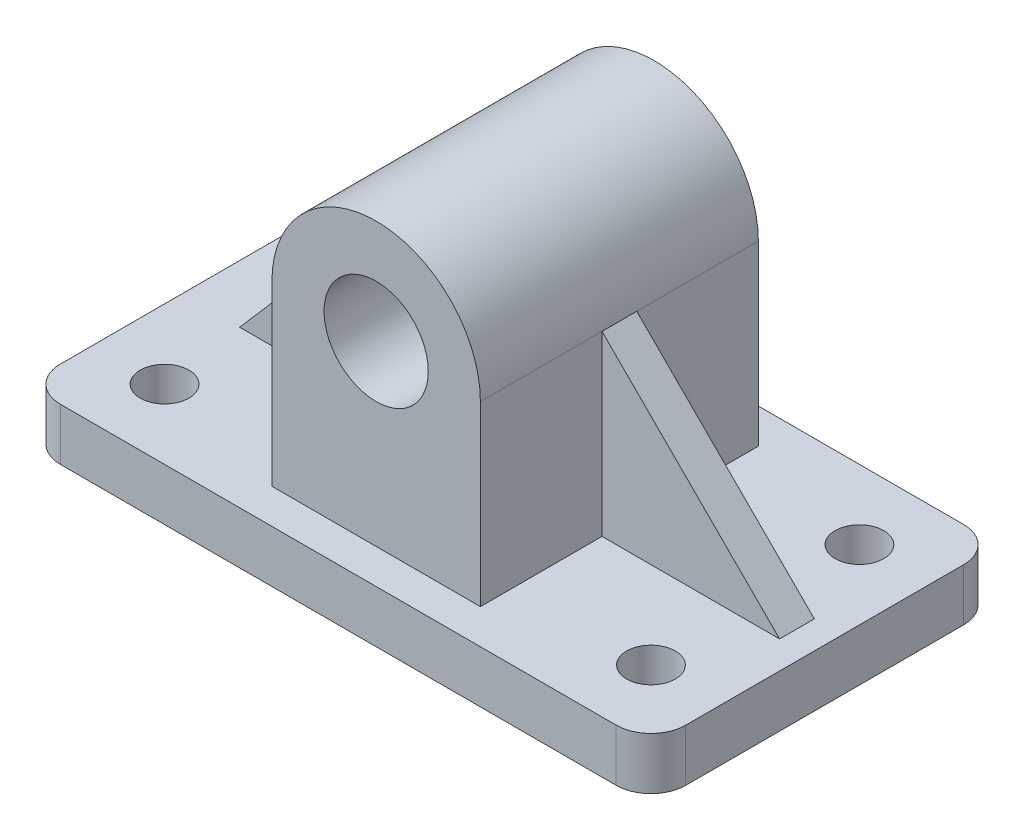
ISO-10303-21;
HEADER;
FILE_DESCRIPTION(('STEP AP214'),'2;1');
FILE_NAME('part.step','',(''),(''),'','','');
FILE_SCHEMA(('AUTOMOTIVE_DESIGN { 1 0 10303 214 1 1 1 1 }'));
ENDSEC;
DATA;
#1=APPLICATION_CONTEXT('core data for automotive mechanical design processes');
#2=APPLICATION_PROTOCOL_DEFINITION('international standard','automotive_design',2000,#1);
#3=PRODUCT_CONTEXT('',#1,'mechanical');
#4=PRODUCT('Part','Part','',(#3));
#5=PRODUCT_RELATED_PRODUCT_CATEGORY('part','',(#4));
#6=PRODUCT_DEFINITION_FORMATION('','',#4);
#7=PRODUCT_DEFINITION_CONTEXT('part definition',#1,'design');
#8=PRODUCT_DEFINITION('design','',#6,#7);
#9=PRODUCT_DEFINITION_SHAPE('','',#8);
#10=(LENGTH_UNIT() NAMED_UNIT(*) SI_UNIT(.MILLI.,.METRE.));
#11=(NAMED_UNIT(*) PLANE_ANGLE_UNIT() SI_UNIT($,.RADIAN.));
#12=(NAMED_UNIT(*) SI_UNIT($,.STERADIAN.) SOLID_ANGLE_UNIT());
#13=UNCERTAINTY_MEASURE_WITH_UNIT(LENGTH_MEASURE(1.E-05),#10,'distance_accuracy_value','');
#14=(GEOMETRIC_REPRESENTATION_CONTEXT(3) GLOBAL_UNCERTAINTY_ASSIGNED_CONTEXT((#13)) GLOBAL_UNIT_ASSIGNED_CONTEXT((#10,
#11,#12)) REPRESENTATION_CONTEXT('',''));
#15=CARTESIAN_POINT('',(0.,0.,0.));
#16=DIRECTION('',(0.,0.,1.));
#17=DIRECTION('',(1.,0.,0.));
#18=AXIS2_PLACEMENT_3D('',#15,#16,#17);
#19=CARTESIAN_POINT('',(120.905881759653,15.,90.));
#20=DIRECTION('',(-1.,0.,0.));
#21=DIRECTION('',(0.,0.,1.));
#22=AXIS2_PLACEMENT_3D('',#19,#20,#21);
#23=PLANE('',#22);
#24=DIRECTION('',(0.,1.,0.));
#25=VECTOR('',#24,1.);
#26=CARTESIAN_POINT('',(120.905881759653,15.,45.));
#27=LINE('',#26,#25);
#28=CARTESIAN_POINT('',(120.905881759653,15.,45.));
#29=VERTEX_POINT('',#28);
#30=CARTESIAN_POINT('',(120.905881759653,66.1058767167039,45.));
#31=VERTEX_POINT('',#30);
#32=EDGE_CURVE('E186',#29,#31,#27,.T.);
#33=ORIENTED_EDGE('',*,*,#32,.F.);
#34=DIRECTION('',(0.,0.,-1.));
#35=VECTOR('',#34,1.);
#36=CARTESIAN_POINT('',(120.905881759653,15.,90.));
#37=LINE('',#36,#35);
#38=CARTESIAN_POINT('',(120.905881759653,15.,10.));
#39=VERTEX_POINT('',#38);
#40=EDGE_CURVE('E196',#29,#39,#37,.T.);
#41=ORIENTED_EDGE('',*,*,#40,.T.);
#42=DIRECTION('',(0.,1.,0.));
#43=VECTOR('',#42,1.);
#44=CARTESIAN_POINT('',(120.905881759653,15.,10.));
#45=LINE('',#44,#43);
#46=CARTESIAN_POINT('',(120.905881759653,66.1058767167039,9.99999999999999));
#47=VERTEX_POINT('',#46);
#48=EDGE_CURVE('E238',#39,#47,#45,.T.);
#49=ORIENTED_EDGE('',*,*,#48,.T.);
#50=DIRECTION('',(0.,0.,-1.));
#51=VECTOR('',#50,1.);
#52=CARTESIAN_POINT('',(120.905881759653,66.1058767167039,90.));
#53=LINE('',#52,#51);
#54=EDGE_CURVE('E245',#31,#47,#53,.T.);
#55=ORIENTED_EDGE('',*,*,#54,.F.);
#56=EDGE_LOOP('',(#33,#41,#49,#55));
#57=FACE_BOUND('',#56,.T.);
#58=ADVANCED_FACE('F44',(#57),#23,.F.);
#59=CARTESIAN_POINT('',(60.9058817596531,66.1058767167039,90.));
#60=DIRECTION('',(1.,0.,0.));
#61=DIRECTION('',(0.,1.,0.));
#62=AXIS2_PLACEMENT_3D('',#59,#60,#61);
#63=PLANE('',#62);
#64=DIRECTION('',(0.,-1.,0.));
#65=VECTOR('',#64,1.);
#66=CARTESIAN_POINT('',(60.9058817596531,66.1058767167039,45.));
#67=LINE('',#66,#65);
#68=CARTESIAN_POINT('',(60.905881759653,66.1058767167037,45.));
#69=VERTEX_POINT('',#68);
#70=CARTESIAN_POINT('',(60.9058817596531,15.,45.));
#71=VERTEX_POINT('',#70);
#72=EDGE_CURVE('E206',#69,#71,#67,.T.);
#73=ORIENTED_EDGE('',*,*,#72,.F.);
#74=DIRECTION('',(0.,0.,-1.));
#75=VECTOR('',#74,1.);
#76=CARTESIAN_POINT('',(60.9058817596531,66.1058767167039,90.));
#77=LINE('',#76,#75);
#78=CARTESIAN_POINT('',(60.9058817596531,66.1058767167039,10.));
#79=VERTEX_POINT('',#78);
#80=EDGE_CURVE('E257',#69,#79,#77,.T.);
#81=ORIENTED_EDGE('',*,*,#80,.T.);
#82=DIRECTION('',(0.,-1.,0.));
#83=VECTOR('',#82,1.);
#84=CARTESIAN_POINT('',(60.9058817596531,66.1058767167039,10.));
#85=LINE('',#84,#83);
#86=CARTESIAN_POINT('',(60.9058817596531,15.,10.));
#87=VERTEX_POINT('',#86);
#88=EDGE_CURVE('E235',#79,#87,#85,.T.);
#89=ORIENTED_EDGE('',*,*,#88,.T.);
#90=DIRECTION('',(0.,0.,-1.));
#91=VECTOR('',#90,1.);
#92=CARTESIAN_POINT('',(60.9058817596531,15.,90.));
#93=LINE('',#92,#91);
#94=EDGE_CURVE('E259',#71,#87,#93,.T.);
#95=ORIENTED_EDGE('',*,*,#94,.F.);
#96=EDGE_LOOP('',(#73,#81,#89,#95));
#97=FACE_BOUND('',#96,.T.);
#98=ADVANCED_FACE('F356',(#97),#63,.F.);
#99=CARTESIAN_POINT('',(0.,15.,100.));
#100=DIRECTION('',(1.,0.,0.));
#101=DIRECTION('',(0.,0.,-1.));
#102=AXIS2_PLACEMENT_3D('',#99,#100,#101);
#103=PLANE('',#102);
#104=DIRECTION('',(0.,0.,-1.));
#105=VECTOR('',#104,1.);
#106=CARTESIAN_POINT('',(0.,15.,100.));
#107=LINE('',#106,#105);
#108=CARTESIAN_POINT('',(0.,15.,90.));
#109=VERTEX_POINT('',#108);
#110=CARTESIAN_POINT('',(0.,15.,9.99999999999999));
#111=VERTEX_POINT('',#110);
#112=EDGE_CURVE('E271',#109,#111,#107,.T.);
#113=ORIENTED_EDGE('',*,*,#112,.T.);
#114=DIRECTION('',(0.,-1.,0.));
#115=VECTOR('',#114,1.);
#116=CARTESIAN_POINT('',(0.,15.,9.99999999999999));
#117=LINE('',#116,#115);
#118=CARTESIAN_POINT('',(0.,0.,9.99999999999999));
#119=VERTEX_POINT('',#118);
#120=EDGE_CURVE('E287',#111,#119,#117,.T.);
#121=ORIENTED_EDGE('',*,*,#120,.T.);
#122=DIRECTION('',(0.,0.,-1.));
#123=VECTOR('',#122,1.);
#124=CARTESIAN_POINT('',(0.,0.,100.));
#125=LINE('',#124,#123);
#126=CARTESIAN_POINT('',(0.,0.,90.));
#127=VERTEX_POINT('',#126);
#128=EDGE_CURVE('E284',#127,#119,#125,.T.);
#129=ORIENTED_EDGE('',*,*,#128,.F.);
#130=DIRECTION('',(0.,-1.,0.));
#131=VECTOR('',#130,1.);
#132=CARTESIAN_POINT('',(0.,15.,90.));
#133=LINE('',#132,#131);
#134=EDGE_CURVE('E286',#127,#109,#133,.F.);
#135=ORIENTED_EDGE('',*,*,#134,.T.);
#136=EDGE_LOOP('',(#113,#121,#129,#135));
#137=FACE_BOUND('',#136,.T.);
#138=ADVANCED_FACE('F331',(#137),#103,.F.);
#139=CARTESIAN_POINT('',(0.,0.,100.));
#140=DIRECTION('',(0.,1.,0.));
#141=DIRECTION('',(0.,0.,1.));
#142=AXIS2_PLACEMENT_3D('',#139,#140,#141);
#143=PLANE('',#142);
#144=CARTESIAN_POINT('',(160.,0.,20.));
#145=DIRECTION('',(0.,1.,0.));
#146=DIRECTION('',(0.,0.,1.));
#147=AXIS2_PLACEMENT_3D('',#144,#145,#146);
#148=CIRCLE('',#147,7.00000000000001);
#149=CARTESIAN_POINT('',(160.,0.,27.));
#150=VERTEX_POINT('',#149);
#151=EDGE_CURVE('E393',#150,#150,#148,.T.);
#152=ORIENTED_EDGE('',*,*,#151,.T.);
#153=EDGE_LOOP('',(#152));
#154=FACE_BOUND('',#153,.T.);
#155=CARTESIAN_POINT('',(160.,0.,80.));
#156=DIRECTION('',(0.,1.,0.));
#157=DIRECTION('',(0.,0.,1.));
#158=AXIS2_PLACEMENT_3D('',#155,#156,#157);
#159=CIRCLE('',#158,6.99999999999998);
#160=CARTESIAN_POINT('',(160.,0.,87.));
#161=VERTEX_POINT('',#160);
#162=EDGE_CURVE('E404',#161,#161,#159,.T.);
#163=ORIENTED_EDGE('',*,*,#162,.T.);
#164=EDGE_LOOP('',(#163));
#165=FACE_BOUND('',#164,.T.);
#166=CARTESIAN_POINT('',(20.,0.,80.));
#167=DIRECTION('',(0.,1.,0.));
#168=DIRECTION('',(0.,0.,1.));
#169=AXIS2_PLACEMENT_3D('',#166,#167,#168);
#170=CIRCLE('',#169,7.);
#171=CARTESIAN_POINT('',(20.,0.,87.));
#172=VERTEX_POINT('',#171);
#173=EDGE_CURVE('E396',#172,#172,#170,.T.);
#174=ORIENTED_EDGE('',*,*,#173,.T.);
#175=EDGE_LOOP('',(#174));
#176=FACE_BOUND('',#175,.T.);
#177=CARTESIAN_POINT('',(20.,0.,20.));
#178=DIRECTION('',(0.,1.,0.));
#179=DIRECTION('',(0.,0.,1.));
#180=AXIS2_PLACEMENT_3D('',#177,#178,#179);
#181=CIRCLE('',#180,7.);
#182=CARTESIAN_POINT('',(20.,0.,27.));
#183=VERTEX_POINT('',#182);
#184=EDGE_CURVE('E194',#183,#183,#181,.T.);
#185=ORIENTED_EDGE('',*,*,#184,.T.);
#186=EDGE_LOOP('',(#185));
#187=FACE_BOUND('',#186,.T.);
#188=ORIENTED_EDGE('',*,*,#128,.T.);
#189=CARTESIAN_POINT('',(10.,0.,9.99999999999999));
#190=DIRECTION('',(0.,1.,0.));
#191=DIRECTION('',(0.,0.,1.));
#192=AXIS2_PLACEMENT_3D('',#189,#190,#191);
#193=CIRCLE('',#192,10.);
#194=CARTESIAN_POINT('',(10.,0.,0.));
#195=VERTEX_POINT('',#194);
#196=EDGE_CURVE('E299',#119,#195,#193,.F.);
#197=ORIENTED_EDGE('',*,*,#196,.T.);
#198=DIRECTION('',(1.,0.,0.));
#199=VECTOR('',#198,1.);
#200=CARTESIAN_POINT('',(0.,0.,0.));
#201=LINE('',#200,#199);
#202=CARTESIAN_POINT('',(170.,0.,0.));
#203=VERTEX_POINT('',#202);
#204=EDGE_CURVE('E263',#195,#203,#201,.T.);
#205=ORIENTED_EDGE('',*,*,#204,.T.);
#206=CARTESIAN_POINT('',(170.,0.,9.99999999999999));
#207=DIRECTION('',(0.,1.,0.));
#208=DIRECTION('',(0.,0.,1.));
#209=AXIS2_PLACEMENT_3D('',#206,#207,#208);
#210=CIRCLE('',#209,10.);
#211=CARTESIAN_POINT('',(180.,0.,9.99999999999999));
#212=VERTEX_POINT('',#211);
#213=EDGE_CURVE('E300',#203,#212,#210,.F.);
#214=ORIENTED_EDGE('',*,*,#213,.T.);
#215=DIRECTION('',(0.,0.,-1.));
#216=VECTOR('',#215,1.);
#217=CARTESIAN_POINT('',(180.,0.,100.));
#218=LINE('',#217,#216);
#219=CARTESIAN_POINT('',(180.,0.,90.));
#220=VERTEX_POINT('',#219);
#221=EDGE_CURVE('E285',#220,#212,#218,.T.);
#222=ORIENTED_EDGE('',*,*,#221,.F.);
#223=CARTESIAN_POINT('',(170.,0.,90.));
#224=DIRECTION('',(0.,1.,0.));
#225=DIRECTION('',(0.,0.,1.));
#226=AXIS2_PLACEMENT_3D('',#223,#224,#225);
#227=CIRCLE('',#226,10.);
#228=CARTESIAN_POINT('',(170.,0.,100.));
#229=VERTEX_POINT('',#228);
#230=EDGE_CURVE('E294',#220,#229,#227,.F.);
#231=ORIENTED_EDGE('',*,*,#230,.T.);
#232=DIRECTION('',(1.,0.,0.));
#233=VECTOR('',#232,1.);
#234=CARTESIAN_POINT('',(0.,0.,100.));
#235=LINE('',#234,#233);
#236=CARTESIAN_POINT('',(10.,0.,100.));
#237=VERTEX_POINT('',#236);
#238=EDGE_CURVE('E268',#237,#229,#235,.T.);
#239=ORIENTED_EDGE('',*,*,#238,.F.);
#240=CARTESIAN_POINT('',(10.,0.,90.));
#241=DIRECTION('',(0.,1.,0.));
#242=DIRECTION('',(0.,0.,1.));
#243=AXIS2_PLACEMENT_3D('',#240,#241,#242);
#244=CIRCLE('',#243,10.);
#245=EDGE_CURVE('E291',#237,#127,#244,.F.);
#246=ORIENTED_EDGE('',*,*,#245,.T.);
#247=EDGE_LOOP('',(#188,#197,#205,#214,#222,#231,#239,#246));
#248=FACE_BOUND('',#247,.T.);
#249=ADVANCED_FACE('F325',(#154,#165,#176,#187,#248),#143,.F.);
#250=CARTESIAN_POINT('',(180.,0.,100.));
#251=DIRECTION('',(-1.,0.,0.));
#252=DIRECTION('',(0.,0.,1.));
#253=AXIS2_PLACEMENT_3D('',#250,#251,#252);
#254=PLANE('',#253);
#255=ORIENTED_EDGE('',*,*,#221,.T.);
#256=DIRECTION('',(0.,1.,0.));
#257=VECTOR('',#256,1.);
#258=CARTESIAN_POINT('',(180.,0.,9.99999999999999));
#259=LINE('',#258,#257);
#260=CARTESIAN_POINT('',(180.,15.,9.99999999999999));
#261=VERTEX_POINT('',#260);
#262=EDGE_CURVE('E312',#212,#261,#259,.T.);
#263=ORIENTED_EDGE('',*,*,#262,.T.);
#264=DIRECTION('',(0.,0.,-1.));
#265=VECTOR('',#264,1.);
#266=CARTESIAN_POINT('',(180.,15.,100.));
#267=LINE('',#266,#265);
#268=CARTESIAN_POINT('',(180.,15.,90.));
#269=VERTEX_POINT('',#268);
#270=EDGE_CURVE('E277',#269,#261,#267,.T.);
#271=ORIENTED_EDGE('',*,*,#270,.F.);
#272=DIRECTION('',(0.,1.,0.));
#273=VECTOR('',#272,1.);
#274=CARTESIAN_POINT('',(180.,0.,90.));
#275=LINE('',#274,#273);
#276=EDGE_CURVE('E311',#269,#220,#275,.F.);
#277=ORIENTED_EDGE('',*,*,#276,.T.);
#278=EDGE_LOOP('',(#255,#263,#271,#277));
#279=FACE_BOUND('',#278,.T.);
#280=ADVANCED_FACE('F346',(#279),#254,.F.);
#281=CARTESIAN_POINT('',(180.,15.,100.));
#282=DIRECTION('',(0.,-1.,0.));
#283=DIRECTION('',(0.,0.,-1.));
#284=AXIS2_PLACEMENT_3D('',#281,#282,#283);
#285=PLANE('',#284);
#286=CARTESIAN_POINT('',(160.,15.,20.));
#287=DIRECTION('',(0.,1.,0.));
#288=DIRECTION('',(0.,0.,1.));
#289=AXIS2_PLACEMENT_3D('',#286,#287,#288);
#290=CIRCLE('',#289,7.00000000000001);
#291=CARTESIAN_POINT('',(160.,15.,27.));
#292=VERTEX_POINT('',#291);
#293=EDGE_CURVE('E406',#292,#292,#290,.T.);
#294=ORIENTED_EDGE('',*,*,#293,.F.);
#295=EDGE_LOOP('',(#294));
#296=FACE_BOUND('',#295,.T.);
#297=CARTESIAN_POINT('',(160.,15.,80.));
#298=DIRECTION('',(0.,1.,0.));
#299=DIRECTION('',(0.,0.,1.));
#300=AXIS2_PLACEMENT_3D('',#297,#298,#299);
#301=CIRCLE('',#300,6.99999999999998);
#302=CARTESIAN_POINT('',(160.,15.,87.));
#303=VERTEX_POINT('',#302);
#304=EDGE_CURVE('E402',#303,#303,#301,.T.);
#305=ORIENTED_EDGE('',*,*,#304,.F.);
#306=EDGE_LOOP('',(#305));
#307=FACE_BOUND('',#306,.T.);
#308=CARTESIAN_POINT('',(20.,15.,80.));
#309=DIRECTION('',(0.,1.,0.));
#310=DIRECTION('',(0.,0.,1.));
#311=AXIS2_PLACEMENT_3D('',#308,#309,#310);
#312=CIRCLE('',#311,7.);
#313=CARTESIAN_POINT('',(20.,15.,87.));
#314=VERTEX_POINT('',#313);
#315=EDGE_CURVE('E394',#314,#314,#312,.T.);
#316=ORIENTED_EDGE('',*,*,#315,.F.);
#317=EDGE_LOOP('',(#316));
#318=FACE_BOUND('',#317,.T.);
#319=CARTESIAN_POINT('',(20.,15.,20.));
#320=DIRECTION('',(0.,1.,0.));
#321=DIRECTION('',(0.,0.,1.));
#322=AXIS2_PLACEMENT_3D('',#319,#320,#321);
#323=CIRCLE('',#322,7.);
#324=CARTESIAN_POINT('',(20.,15.,27.));
#325=VERTEX_POINT('',#324);
#326=EDGE_CURVE('E391',#325,#325,#323,.T.);
#327=ORIENTED_EDGE('',*,*,#326,.F.);
#328=EDGE_LOOP('',(#327));
#329=FACE_BOUND('',#328,.T.);
#330=DIRECTION('',(-1.,0.,0.));
#331=VECTOR('',#330,1.);
#332=CARTESIAN_POINT('',(180.,15.,0.));
#333=LINE('',#332,#331);
#334=CARTESIAN_POINT('',(170.,15.,0.));
#335=VERTEX_POINT('',#334);
#336=CARTESIAN_POINT('',(10.0000000000001,15.,0.));
#337=VERTEX_POINT('',#336);
#338=EDGE_CURVE('E267',#335,#337,#333,.T.);
#339=ORIENTED_EDGE('',*,*,#338,.T.);
#340=CARTESIAN_POINT('',(10.,15.,9.99999999999999));
#341=DIRECTION('',(0.,-1.,0.));
#342=DIRECTION('',(0.,0.,-1.));
#343=AXIS2_PLACEMENT_3D('',#340,#341,#342);
#344=CIRCLE('',#343,10.);
#345=EDGE_CURVE('E307',#337,#111,#344,.F.);
#346=ORIENTED_EDGE('',*,*,#345,.T.);
#347=ORIENTED_EDGE('',*,*,#112,.F.);
#348=CARTESIAN_POINT('',(10.,15.,90.));
#349=DIRECTION('',(0.,-1.,0.));
#350=DIRECTION('',(0.,0.,-1.));
#351=AXIS2_PLACEMENT_3D('',#348,#349,#350);
#352=CIRCLE('',#351,10.);
#353=CARTESIAN_POINT('',(10.0000000000001,15.,100.));
#354=VERTEX_POINT('',#353);
#355=EDGE_CURVE('E304',#109,#354,#352,.F.);
#356=ORIENTED_EDGE('',*,*,#355,.T.);
#357=DIRECTION('',(-1.,0.,0.));
#358=VECTOR('',#357,1.);
#359=CARTESIAN_POINT('',(180.,15.,100.));
#360=LINE('',#359,#358);
#361=CARTESIAN_POINT('',(170.,15.,100.));
#362=VERTEX_POINT('',#361);
#363=EDGE_CURVE('E269',#362,#354,#360,.T.);
#364=ORIENTED_EDGE('',*,*,#363,.F.);
#365=CARTESIAN_POINT('',(170.,15.,90.));
#366=DIRECTION('',(0.,-1.,0.));
#367=DIRECTION('',(0.,0.,-1.));
#368=AXIS2_PLACEMENT_3D('',#365,#366,#367);
#369=CIRCLE('',#368,10.);
#370=EDGE_CURVE('E67',#362,#269,#369,.F.);
#371=ORIENTED_EDGE('',*,*,#370,.T.);
#372=ORIENTED_EDGE('',*,*,#270,.T.);
#373=CARTESIAN_POINT('',(170.,15.,9.99999999999999));
#374=DIRECTION('',(0.,-1.,0.));
#375=DIRECTION('',(0.,0.,-1.));
#376=AXIS2_PLACEMENT_3D('',#373,#374,#375);
#377=CIRCLE('',#376,10.);
#378=EDGE_CURVE('E58',#261,#335,#377,.F.);
#379=ORIENTED_EDGE('',*,*,#378,.T.);
#380=EDGE_LOOP('',(#339,#346,#347,#356,#364,#371,#372,#379));
#381=FACE_BOUND('',#380,.T.);
#382=DIRECTION('',(-1.,0.,0.));
#383=VECTOR('',#382,1.);
#384=CARTESIAN_POINT('',(180.,15.,55.));
#385=LINE('',#384,#383);
#386=CARTESIAN_POINT('',(60.9058817596531,15.,55.));
#387=VERTEX_POINT('',#386);
#388=CARTESIAN_POINT('',(16.6235774681034,15.,55.));
#389=VERTEX_POINT('',#388);
#390=EDGE_CURVE('E220',#387,#389,#385,.T.);
#391=ORIENTED_EDGE('',*,*,#390,.T.);
#392=DIRECTION('',(0.,0.,-1.));
#393=VECTOR('',#392,1.);
#394=CARTESIAN_POINT('',(16.6235774681034,15.,100.));
#395=LINE('',#394,#393);
#396=CARTESIAN_POINT('',(16.6235774681034,15.,45.));
#397=VERTEX_POINT('',#396);
#398=EDGE_CURVE('E218',#389,#397,#395,.T.);
#399=ORIENTED_EDGE('',*,*,#398,.T.);
#400=DIRECTION('',(-1.,0.,0.));
#401=VECTOR('',#400,1.);
#402=CARTESIAN_POINT('',(180.,15.,45.));
#403=LINE('',#402,#401);
#404=EDGE_CURVE('E214',#71,#397,#403,.T.);
#405=ORIENTED_EDGE('',*,*,#404,.F.);
#406=ORIENTED_EDGE('',*,*,#94,.T.);
#407=DIRECTION('',(1.,0.,0.));
#408=VECTOR('',#407,1.);
#409=CARTESIAN_POINT('',(60.9058817596531,15.,10.));
#410=LINE('',#409,#408);
#411=EDGE_CURVE('E244',#87,#39,#410,.T.);
#412=ORIENTED_EDGE('',*,*,#411,.T.);
#413=ORIENTED_EDGE('',*,*,#40,.F.);
#414=DIRECTION('',(-1.,0.,0.));
#415=VECTOR('',#414,1.);
#416=CARTESIAN_POINT('',(180.,15.,45.));
#417=LINE('',#416,#415);
#418=CARTESIAN_POINT('',(172.011758476358,15.,45.));
#419=VERTEX_POINT('',#418);
#420=EDGE_CURVE('E190',#419,#29,#417,.T.);
#421=ORIENTED_EDGE('',*,*,#420,.F.);
#422=DIRECTION('',(0.,0.,-1.));
#423=VECTOR('',#422,1.);
#424=CARTESIAN_POINT('',(172.011758476358,15.,100.));
#425=LINE('',#424,#423);
#426=CARTESIAN_POINT('',(172.011758476358,15.,55.));
#427=VERTEX_POINT('',#426);
#428=EDGE_CURVE('E175',#419,#427,#425,.F.);
#429=ORIENTED_EDGE('',*,*,#428,.T.);
#430=DIRECTION('',(-1.,0.,0.));
#431=VECTOR('',#430,1.);
#432=CARTESIAN_POINT('',(180.,15.,55.));
#433=LINE('',#432,#431);
#434=CARTESIAN_POINT('',(120.905881759653,15.,55.));
#435=VERTEX_POINT('',#434);
#436=EDGE_CURVE('E182',#427,#435,#433,.T.);
#437=ORIENTED_EDGE('',*,*,#436,.T.);
#438=CARTESIAN_POINT('',(120.905881759653,15.,90.));
#439=VERTEX_POINT('',#438);
#440=EDGE_CURVE('E254',#439,#435,#37,.T.);
#441=ORIENTED_EDGE('',*,*,#440,.F.);
#442=DIRECTION('',(1.,0.,0.));
#443=VECTOR('',#442,1.);
#444=CARTESIAN_POINT('',(60.9058817596531,15.,90.));
#445=LINE('',#444,#443);
#446=CARTESIAN_POINT('',(60.9058817596531,15.,90.));
#447=VERTEX_POINT('',#446);
#448=EDGE_CURVE('E240',#447,#439,#445,.T.);
#449=ORIENTED_EDGE('',*,*,#448,.F.);
#450=EDGE_CURVE('E256',#447,#387,#93,.T.);
#451=ORIENTED_EDGE('',*,*,#450,.T.);
#452=EDGE_LOOP('',(#391,#399,#405,#406,#412,#413,#421,#429,#437,#441,#449,#451));
#453=FACE_BOUND('',#452,.T.);
#454=ADVANCED_FACE('F193',(#296,#307,#318,#329,#381,#453),#285,.F.);
#455=CARTESIAN_POINT('',(0.,0.,100.));
#456=DIRECTION('',(0.,0.,1.));
#457=DIRECTION('',(1.,0.,0.));
#458=AXIS2_PLACEMENT_3D('',#455,#456,#457);
#459=PLANE('',#458);
#460=ORIENTED_EDGE('',*,*,#238,.T.);
#461=DIRECTION('',(0.,1.,0.));
#462=VECTOR('',#461,1.);
#463=CARTESIAN_POINT('',(170.,15.,100.));
#464=LINE('',#463,#462);
#465=EDGE_CURVE('E12',#229,#362,#464,.T.);
#466=ORIENTED_EDGE('',*,*,#465,.T.);
#467=ORIENTED_EDGE('',*,*,#363,.T.);
#468=DIRECTION('',(0.,-1.,0.));
#469=VECTOR('',#468,1.);
#470=CARTESIAN_POINT('',(10.,0.,100.));
#471=LINE('',#470,#469);
#472=EDGE_CURVE('E52',#354,#237,#471,.T.);
#473=ORIENTED_EDGE('',*,*,#472,.T.);
#474=EDGE_LOOP('',(#460,#466,#467,#473));
#475=FACE_BOUND('',#474,.T.);
#476=ADVANCED_FACE('F319',(#475),#459,.T.);
#477=CARTESIAN_POINT('',(0.,0.,0.));
#478=DIRECTION('',(0.,0.,1.));
#479=DIRECTION('',(1.,0.,0.));
#480=AXIS2_PLACEMENT_3D('',#477,#478,#479);
#481=PLANE('',#480);
#482=ORIENTED_EDGE('',*,*,#204,.F.);
#483=DIRECTION('',(0.,-1.,0.));
#484=VECTOR('',#483,1.);
#485=CARTESIAN_POINT('',(10.,0.,0.));
#486=LINE('',#485,#484);
#487=EDGE_CURVE('E303',#195,#337,#486,.F.);
#488=ORIENTED_EDGE('',*,*,#487,.T.);
#489=ORIENTED_EDGE('',*,*,#338,.F.);
#490=DIRECTION('',(0.,1.,0.));
#491=VECTOR('',#490,1.);
#492=CARTESIAN_POINT('',(170.,0.,0.));
#493=LINE('',#492,#491);
#494=EDGE_CURVE('E301',#335,#203,#493,.F.);
#495=ORIENTED_EDGE('',*,*,#494,.T.);
#496=EDGE_LOOP('',(#482,#488,#489,#495));
#497=FACE_BOUND('',#496,.T.);
#498=ADVANCED_FACE('F338',(#497),#481,.F.);
#499=CARTESIAN_POINT('',(60.9058817596531,66.1058767167039,90.));
#500=VERTEX_POINT('',#499);
#501=CARTESIAN_POINT('',(60.9058817596531,66.1058767167039,55.));
#502=VERTEX_POINT('',#501);
#503=EDGE_CURVE('E261',#500,#502,#77,.T.);
#504=ORIENTED_EDGE('',*,*,#503,.T.);
#505=DIRECTION('',(0.,-1.,0.));
#506=VECTOR('',#505,1.);
#507=CARTESIAN_POINT('',(60.9058817596531,66.1058767167039,55.));
#508=LINE('',#507,#506);
#509=EDGE_CURVE('E213',#502,#387,#508,.T.);
#510=ORIENTED_EDGE('',*,*,#509,.T.);
#511=ORIENTED_EDGE('',*,*,#450,.F.);
#512=DIRECTION('',(0.,-1.,0.));
#513=VECTOR('',#512,1.);
#514=CARTESIAN_POINT('',(60.9058817596531,66.1058767167039,90.));
#515=LINE('',#514,#513);
#516=EDGE_CURVE('E232',#500,#447,#515,.T.);
#517=ORIENTED_EDGE('',*,*,#516,.F.);
#518=EDGE_LOOP('',(#504,#510,#511,#517));
#519=FACE_BOUND('',#518,.T.);
#520=ADVANCED_FACE('F367',(#519),#63,.F.);
#521=ORIENTED_EDGE('',*,*,#440,.T.);
#522=DIRECTION('',(0.,1.,0.));
#523=VECTOR('',#522,1.);
#524=CARTESIAN_POINT('',(120.905881759653,15.,55.));
#525=LINE('',#524,#523);
#526=CARTESIAN_POINT('',(120.905881759653,66.1058767167039,55.));
#527=VERTEX_POINT('',#526);
#528=EDGE_CURVE('E200',#435,#527,#525,.T.);
#529=ORIENTED_EDGE('',*,*,#528,.T.);
#530=CARTESIAN_POINT('',(120.905881759653,66.1058767167039,90.));
#531=VERTEX_POINT('',#530);
#532=EDGE_CURVE('E248',#531,#527,#53,.T.);
#533=ORIENTED_EDGE('',*,*,#532,.F.);
#534=DIRECTION('',(0.,1.,0.));
#535=VECTOR('',#534,1.);
#536=CARTESIAN_POINT('',(120.905881759653,15.,90.));
#537=LINE('',#536,#535);
#538=EDGE_CURVE('E239',#439,#531,#537,.T.);
#539=ORIENTED_EDGE('',*,*,#538,.F.);
#540=EDGE_LOOP('',(#521,#529,#533,#539));
#541=FACE_BOUND('',#540,.T.);
#542=ADVANCED_FACE('F363',(#541),#23,.F.);
#543=CARTESIAN_POINT('',(0.,0.,90.));
#544=DIRECTION('',(0.,0.,1.));
#545=DIRECTION('',(1.,0.,0.));
#546=AXIS2_PLACEMENT_3D('',#543,#544,#545);
#547=PLANE('',#546);
#548=CARTESIAN_POINT('',(90.9058817596531,66.1058767167039,90.));
#549=DIRECTION('',(0.,0.,1.));
#550=DIRECTION('',(1.,0.,0.));
#551=AXIS2_PLACEMENT_3D('',#548,#549,#550);
#552=CIRCLE('',#551,15.);
#553=CARTESIAN_POINT('',(105.905881759653,66.1058767167039,90.));
#554=VERTEX_POINT('',#553);
#555=EDGE_CURVE('E225',#554,#554,#552,.T.);
#556=ORIENTED_EDGE('',*,*,#555,.F.);
#557=EDGE_LOOP('',(#556));
#558=FACE_BOUND('',#557,.T.);
#559=ORIENTED_EDGE('',*,*,#538,.T.);
#560=CARTESIAN_POINT('',(90.9058817596531,66.1058767167039,90.));
#561=DIRECTION('',(0.,0.,1.));
#562=DIRECTION('',(1.,0.,0.));
#563=AXIS2_PLACEMENT_3D('',#560,#561,#562);
#564=CIRCLE('',#563,30.);
#565=EDGE_CURVE('E228',#531,#500,#564,.T.);
#566=ORIENTED_EDGE('',*,*,#565,.T.);
#567=ORIENTED_EDGE('',*,*,#516,.T.);
#568=ORIENTED_EDGE('',*,*,#448,.T.);
#569=EDGE_LOOP('',(#559,#566,#567,#568));
#570=FACE_BOUND('',#569,.T.);
#571=ADVANCED_FACE('F371',(#558,#570),#547,.T.);
#572=CARTESIAN_POINT('',(0.,0.,10.));
#573=DIRECTION('',(0.,0.,1.));
#574=DIRECTION('',(1.,0.,0.));
#575=AXIS2_PLACEMENT_3D('',#572,#573,#574);
#576=PLANE('',#575);
#577=CARTESIAN_POINT('',(90.9058817596531,66.1058767167039,9.99999999999999));
#578=DIRECTION('',(0.,0.,1.));
#579=DIRECTION('',(1.,0.,0.));
#580=AXIS2_PLACEMENT_3D('',#577,#578,#579);
#581=CIRCLE('',#580,15.);
#582=CARTESIAN_POINT('',(105.905881759653,66.1058767167039,9.99999999999999));
#583=VERTEX_POINT('',#582);
#584=EDGE_CURVE('E221',#583,#583,#581,.T.);
#585=ORIENTED_EDGE('',*,*,#584,.T.);
#586=EDGE_LOOP('',(#585));
#587=FACE_BOUND('',#586,.T.);
#588=ORIENTED_EDGE('',*,*,#88,.F.);
#589=CARTESIAN_POINT('',(90.9058817596531,66.1058767167039,9.99999999999999));
#590=DIRECTION('',(0.,0.,1.));
#591=DIRECTION('',(1.,0.,0.));
#592=AXIS2_PLACEMENT_3D('',#589,#590,#591);
#593=CIRCLE('',#592,30.);
#594=EDGE_CURVE('E230',#47,#79,#593,.T.);
#595=ORIENTED_EDGE('',*,*,#594,.F.);
#596=ORIENTED_EDGE('',*,*,#48,.F.);
#597=ORIENTED_EDGE('',*,*,#411,.F.);
#598=EDGE_LOOP('',(#588,#595,#596,#597));
#599=FACE_BOUND('',#598,.T.);
#600=ADVANCED_FACE('F380',(#587,#599),#576,.F.);
#601=CARTESIAN_POINT('',(90.9058817596531,66.1058767167039,9.99999999999999));
#602=DIRECTION('',(0.,0.,1.));
#603=DIRECTION('',(1.,0.,0.));
#604=AXIS2_PLACEMENT_3D('',#601,#602,#603);
#605=CYLINDRICAL_SURFACE('',#604,15.);
#606=ORIENTED_EDGE('',*,*,#555,.T.);
#607=EDGE_LOOP('',(#606));
#608=FACE_BOUND('',#607,.T.);
#609=ORIENTED_EDGE('',*,*,#584,.F.);
#610=EDGE_LOOP('',(#609));
#611=FACE_BOUND('',#610,.T.);
#612=ADVANCED_FACE('F458',(#608,#611),#605,.F.);
#613=CARTESIAN_POINT('',(90.9058817596531,66.1058767167039,9.99999999999999));
#614=DIRECTION('',(0.,0.,1.));
#615=DIRECTION('',(1.,0.,0.));
#616=AXIS2_PLACEMENT_3D('',#613,#614,#615);
#617=CYLINDRICAL_SURFACE('',#616,30.);
#618=EDGE_CURVE('E264',#502,#69,#77,.T.);
#619=ORIENTED_EDGE('',*,*,#618,.F.);
#620=ORIENTED_EDGE('',*,*,#503,.F.);
#621=ORIENTED_EDGE('',*,*,#565,.F.);
#622=ORIENTED_EDGE('',*,*,#532,.T.);
#623=EDGE_CURVE('E255',#527,#31,#53,.T.);
#624=ORIENTED_EDGE('',*,*,#623,.T.);
#625=ORIENTED_EDGE('',*,*,#54,.T.);
#626=ORIENTED_EDGE('',*,*,#594,.T.);
#627=ORIENTED_EDGE('',*,*,#80,.F.);
#628=EDGE_LOOP('',(#619,#620,#621,#622,#624,#625,#626,#627));
#629=FACE_BOUND('',#628,.T.);
#630=ADVANCED_FACE('F460',(#629),#617,.T.);
#631=CARTESIAN_POINT('',(60.9058817596531,66.1058767167037,50.));
#632=DIRECTION('',(-0.755758283387336,0.654850683050287,0.));
#633=DIRECTION('',(-0.654850683050287,-0.755758283387336,0.));
#634=AXIS2_PLACEMENT_3D('',#631,#632,#633);
#635=PLANE('',#634);
#636=ORIENTED_EDGE('',*,*,#398,.F.);
#637=DIRECTION('',(-0.654850683050287,-0.755758283387336,0.));
#638=VECTOR('',#637,1.);
#639=CARTESIAN_POINT('',(60.9058817596531,66.1058767167037,55.));
#640=LINE('',#639,#638);
#641=EDGE_CURVE('E202',#502,#389,#640,.T.);
#642=ORIENTED_EDGE('',*,*,#641,.F.);
#643=ORIENTED_EDGE('',*,*,#618,.T.);
#644=DIRECTION('',(-0.654850683050287,-0.755758283387336,0.));
#645=VECTOR('',#644,1.);
#646=CARTESIAN_POINT('',(60.9058817596531,66.1058767167037,45.));
#647=LINE('',#646,#645);
#648=EDGE_CURVE('E185',#69,#397,#647,.T.);
#649=ORIENTED_EDGE('',*,*,#648,.T.);
#650=EDGE_LOOP('',(#636,#642,#643,#649));
#651=FACE_BOUND('',#650,.T.);
#652=ADVANCED_FACE('F454',(#651),#635,.T.);
#653=CARTESIAN_POINT('',(90.,48.052938358352,55.));
#654=DIRECTION('',(0.,0.,1.));
#655=DIRECTION('',(1.,0.,0.));
#656=AXIS2_PLACEMENT_3D('',#653,#654,#655);
#657=PLANE('',#656);
#658=ORIENTED_EDGE('',*,*,#390,.F.);
#659=ORIENTED_EDGE('',*,*,#509,.F.);
#660=ORIENTED_EDGE('',*,*,#641,.T.);
#661=EDGE_LOOP('',(#658,#659,#660));
#662=FACE_BOUND('',#661,.T.);
#663=ADVANCED_FACE('F449',(#662),#657,.T.);
#664=CARTESIAN_POINT('',(90.,48.052938358352,45.));
#665=DIRECTION('',(0.,0.,1.));
#666=DIRECTION('',(1.,0.,0.));
#667=AXIS2_PLACEMENT_3D('',#664,#665,#666);
#668=PLANE('',#667);
#669=ORIENTED_EDGE('',*,*,#72,.T.);
#670=ORIENTED_EDGE('',*,*,#404,.T.);
#671=ORIENTED_EDGE('',*,*,#648,.F.);
#672=EDGE_LOOP('',(#669,#670,#671));
#673=FACE_BOUND('',#672,.T.);
#674=ADVANCED_FACE('F450',(#673),#668,.F.);
#675=CARTESIAN_POINT('',(120.905881759653,66.1058767167039,50.));
#676=DIRECTION('',(-0.707106781186539,-0.707106781186556,0.));
#677=DIRECTION('',(0.707106781186556,-0.707106781186539,0.));
#678=AXIS2_PLACEMENT_3D('',#675,#676,#677);
#679=PLANE('',#678);
#680=ORIENTED_EDGE('',*,*,#428,.F.);
#681=DIRECTION('',(0.707106781186556,-0.707106781186539,0.));
#682=VECTOR('',#681,1.);
#683=CARTESIAN_POINT('',(120.905881759653,66.1058767167039,45.));
#684=LINE('',#683,#682);
#685=EDGE_CURVE('E174',#31,#419,#684,.T.);
#686=ORIENTED_EDGE('',*,*,#685,.F.);
#687=ORIENTED_EDGE('',*,*,#623,.F.);
#688=DIRECTION('',(0.707106781186556,-0.707106781186539,0.));
#689=VECTOR('',#688,1.);
#690=CARTESIAN_POINT('',(120.905881759653,66.1058767167039,55.));
#691=LINE('',#690,#689);
#692=EDGE_CURVE('E178',#527,#427,#691,.T.);
#693=ORIENTED_EDGE('',*,*,#692,.T.);
#694=EDGE_LOOP('',(#680,#686,#687,#693));
#695=FACE_BOUND('',#694,.T.);
#696=ADVANCED_FACE('F172',(#695),#679,.F.);
#697=CARTESIAN_POINT('',(90.,48.052938358352,55.));
#698=DIRECTION('',(0.,0.,1.));
#699=DIRECTION('',(1.,0.,0.));
#700=AXIS2_PLACEMENT_3D('',#697,#698,#699);
#701=PLANE('',#700);
#702=ORIENTED_EDGE('',*,*,#436,.F.);
#703=ORIENTED_EDGE('',*,*,#692,.F.);
#704=ORIENTED_EDGE('',*,*,#528,.F.);
#705=EDGE_LOOP('',(#702,#703,#704));
#706=FACE_BOUND('',#705,.T.);
#707=ADVANCED_FACE('F386',(#706),#701,.T.);
#708=CARTESIAN_POINT('',(90.,48.052938358352,45.));
#709=DIRECTION('',(0.,0.,1.));
#710=DIRECTION('',(1.,0.,0.));
#711=AXIS2_PLACEMENT_3D('',#708,#709,#710);
#712=PLANE('',#711);
#713=ORIENTED_EDGE('',*,*,#685,.T.);
#714=ORIENTED_EDGE('',*,*,#420,.T.);
#715=ORIENTED_EDGE('',*,*,#32,.T.);
#716=EDGE_LOOP('',(#713,#714,#715));
#717=FACE_BOUND('',#716,.T.);
#718=ADVANCED_FACE('F187',(#717),#712,.F.);
#719=CARTESIAN_POINT('',(20.,-65.,20.));
#720=DIRECTION('',(0.,1.,0.));
#721=DIRECTION('',(0.,0.,1.));
#722=AXIS2_PLACEMENT_3D('',#719,#720,#721);
#723=CYLINDRICAL_SURFACE('',#722,7.);
#724=ORIENTED_EDGE('',*,*,#326,.T.);
#725=EDGE_LOOP('',(#724));
#726=FACE_BOUND('',#725,.T.);
#727=ORIENTED_EDGE('',*,*,#184,.F.);
#728=EDGE_LOOP('',(#727));
#729=FACE_BOUND('',#728,.T.);
#730=ADVANCED_FACE('F430',(#726,#729),#723,.F.);
#731=CARTESIAN_POINT('',(20.,0.,80.));
#732=DIRECTION('',(0.,1.,0.));
#733=DIRECTION('',(0.,0.,1.));
#734=AXIS2_PLACEMENT_3D('',#731,#732,#733);
#735=CYLINDRICAL_SURFACE('',#734,7.);
#736=ORIENTED_EDGE('',*,*,#173,.F.);
#737=EDGE_LOOP('',(#736));
#738=FACE_BOUND('',#737,.T.);
#739=ORIENTED_EDGE('',*,*,#315,.T.);
#740=EDGE_LOOP('',(#739));
#741=FACE_BOUND('',#740,.T.);
#742=ADVANCED_FACE('F427',(#738,#741),#735,.F.);
#743=CARTESIAN_POINT('',(160.,0.,80.));
#744=DIRECTION('',(0.,1.,0.));
#745=DIRECTION('',(0.,0.,1.));
#746=AXIS2_PLACEMENT_3D('',#743,#744,#745);
#747=CYLINDRICAL_SURFACE('',#746,6.99999999999998);
#748=ORIENTED_EDGE('',*,*,#162,.F.);
#749=EDGE_LOOP('',(#748));
#750=FACE_BOUND('',#749,.T.);
#751=ORIENTED_EDGE('',*,*,#304,.T.);
#752=EDGE_LOOP('',(#751));
#753=FACE_BOUND('',#752,.T.);
#754=ADVANCED_FACE('F420',(#750,#753),#747,.F.);
#755=CARTESIAN_POINT('',(160.,0.,20.));
#756=DIRECTION('',(0.,1.,0.));
#757=DIRECTION('',(0.,0.,1.));
#758=AXIS2_PLACEMENT_3D('',#755,#756,#757);
#759=CYLINDRICAL_SURFACE('',#758,7.00000000000001);
#760=ORIENTED_EDGE('',*,*,#151,.F.);
#761=EDGE_LOOP('',(#760));
#762=FACE_BOUND('',#761,.T.);
#763=ORIENTED_EDGE('',*,*,#293,.T.);
#764=EDGE_LOOP('',(#763));
#765=FACE_BOUND('',#764,.T.);
#766=ADVANCED_FACE('F413',(#762,#765),#759,.F.);
#767=CARTESIAN_POINT('',(10.,15.,9.99999999999999));
#768=DIRECTION('',(0.,-1.,0.));
#769=DIRECTION('',(0.,0.,-1.));
#770=AXIS2_PLACEMENT_3D('',#767,#768,#769);
#771=CYLINDRICAL_SURFACE('',#770,10.);
#772=ORIENTED_EDGE('',*,*,#345,.F.);
#773=ORIENTED_EDGE('',*,*,#487,.F.);
#774=ORIENTED_EDGE('',*,*,#196,.F.);
#775=ORIENTED_EDGE('',*,*,#120,.F.);
#776=EDGE_LOOP('',(#772,#773,#774,#775));
#777=FACE_BOUND('',#776,.T.);
#778=ADVANCED_FACE('F345',(#777),#771,.T.);
#779=CARTESIAN_POINT('',(170.,0.,9.99999999999999));
#780=DIRECTION('',(0.,1.,0.));
#781=DIRECTION('',(0.,0.,1.));
#782=AXIS2_PLACEMENT_3D('',#779,#780,#781);
#783=CYLINDRICAL_SURFACE('',#782,10.);
#784=ORIENTED_EDGE('',*,*,#213,.F.);
#785=ORIENTED_EDGE('',*,*,#494,.F.);
#786=ORIENTED_EDGE('',*,*,#378,.F.);
#787=ORIENTED_EDGE('',*,*,#262,.F.);
#788=EDGE_LOOP('',(#784,#785,#786,#787));
#789=FACE_BOUND('',#788,.T.);
#790=ADVANCED_FACE('F343',(#789),#783,.T.);
#791=CARTESIAN_POINT('',(170.,0.,90.));
#792=DIRECTION('',(0.,-1.,0.));
#793=DIRECTION('',(0.,0.,-1.));
#794=AXIS2_PLACEMENT_3D('',#791,#792,#793);
#795=CYLINDRICAL_SURFACE('',#794,10.);
#796=ORIENTED_EDGE('',*,*,#230,.F.);
#797=ORIENTED_EDGE('',*,*,#276,.F.);
#798=ORIENTED_EDGE('',*,*,#370,.F.);
#799=ORIENTED_EDGE('',*,*,#465,.F.);
#800=EDGE_LOOP('',(#796,#797,#798,#799));
#801=FACE_BOUND('',#800,.T.);
#802=ADVANCED_FACE('F328',(#801),#795,.T.);
#803=CARTESIAN_POINT('',(10.,0.,90.));
#804=DIRECTION('',(0.,1.,0.));
#805=DIRECTION('',(0.,0.,1.));
#806=AXIS2_PLACEMENT_3D('',#803,#804,#805);
#807=CYLINDRICAL_SURFACE('',#806,10.);
#808=ORIENTED_EDGE('',*,*,#355,.F.);
#809=ORIENTED_EDGE('',*,*,#134,.F.);
#810=ORIENTED_EDGE('',*,*,#245,.F.);
#811=ORIENTED_EDGE('',*,*,#472,.F.);
#812=EDGE_LOOP('',(#808,#809,#810,#811));
#813=FACE_BOUND('',#812,.T.);
#814=ADVANCED_FACE('F50',(#813),#807,.T.);
#815=CLOSED_SHELL('',(#58,#98,#138,#249,#280,#454,#476,#498,#520,#542,#571,#600,#612,#630,#652,
#663,#674,#696,#707,#718,#730,#742,#754,#766,#778,#790,#802,#814));
#816=MANIFOLD_SOLID_BREP('B2',#815);
#817=ADVANCED_BREP_SHAPE_REPRESENTATION('',(#18,#816),#14);
#818=SHAPE_DEFINITION_REPRESENTATION(#9,#817);
ENDSEC;
END-ISO-10303-21;
